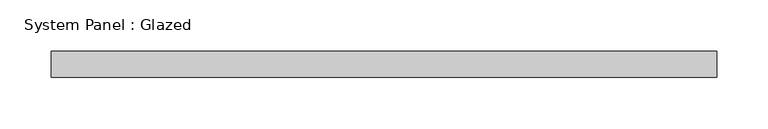
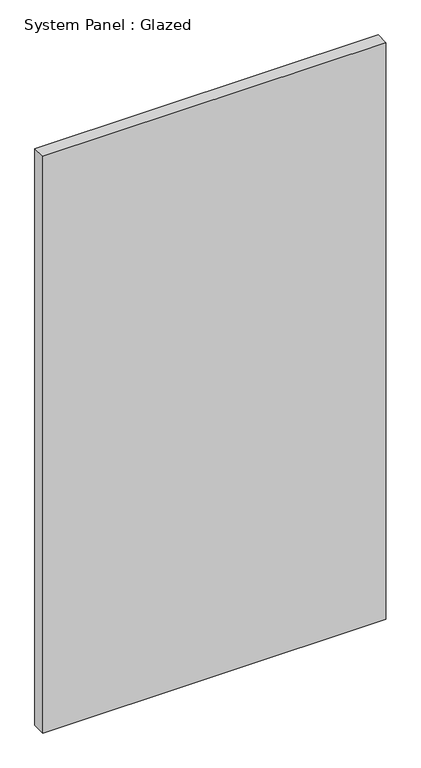
"""IFC4 building model written with IfcOpenShell, lengths in millimetres: plate geometry, System Panel : Glazed."""

from ifc_helpers import new_model, si_unit, origin, origin_with_axes, place, context, project, spatial, polyline, outline, extrude, source, transform, mapped, element, save


def system_panel_glazed_d08d7fb2(model_context):
    return source(origin(), model_context, "Body", "SweptSolid", [
        extrude(outline(polyline([(325.2270709, 19.05), (-325.2270709, 19.05), (-325.2270709, 44.45), (325.2270709, 44.45), (325.2270709, 19.05)])), origin_with_axes(), (0.0, 0.0, 1.0), 1155.7),
    ])


if __name__ == "__main__":
    model = new_model("IFC4")
    model_context = context("Model", 3, world=origin())
    ifc_project = project(units=[si_unit("LENGTHUNIT", "METRE", prefix="MILLI")], contexts=[model_context])
    site = spatial("IfcSite", under=ifc_project)
    building = spatial("IfcBuilding", under=site)
    placement = place(None, origin())
    system_panel_glazed_shape = system_panel_glazed_d08d7fb2(model_context)
    element("IfcPlate", 1, ObjectType="System Panel : Glazed", at=placement, inside=building, context=model_context, shape_type="MappedRepresentation", body=[
        mapped(system_panel_glazed_shape, transform((0.0, 0.0, 0.0), x_axis=(1.0, 0.0, 0.0), y_axis=(0.0, 1.0, 0.0), z_axis=(0.0, 0.0, 1.0))),
    ])
    save(model, "model.ifc")

# Revit data of these elements
# Type "System Panel : Glazed"
#   Construction Type Id = "GSP4R"
#   Analytic Construction = "1/8 in Pilkington single glazing"
#   Visual Light Transmittance = 0.9
#   Solar Heat Gain Coefficient = 0.86
#   Heat Transfer Coefficient (U) = 1.18115 BTU/(h·ft²·°F)
# Element 1 (IfcPlate, "System Panel : Glazed")
#   Materials on its faces: "Glass"
# Materials
#   "Glass": class "Glass", colour RGB 0 128 192, transparency 0.75, Description = "Soda Lime Glass", Cost = 0
